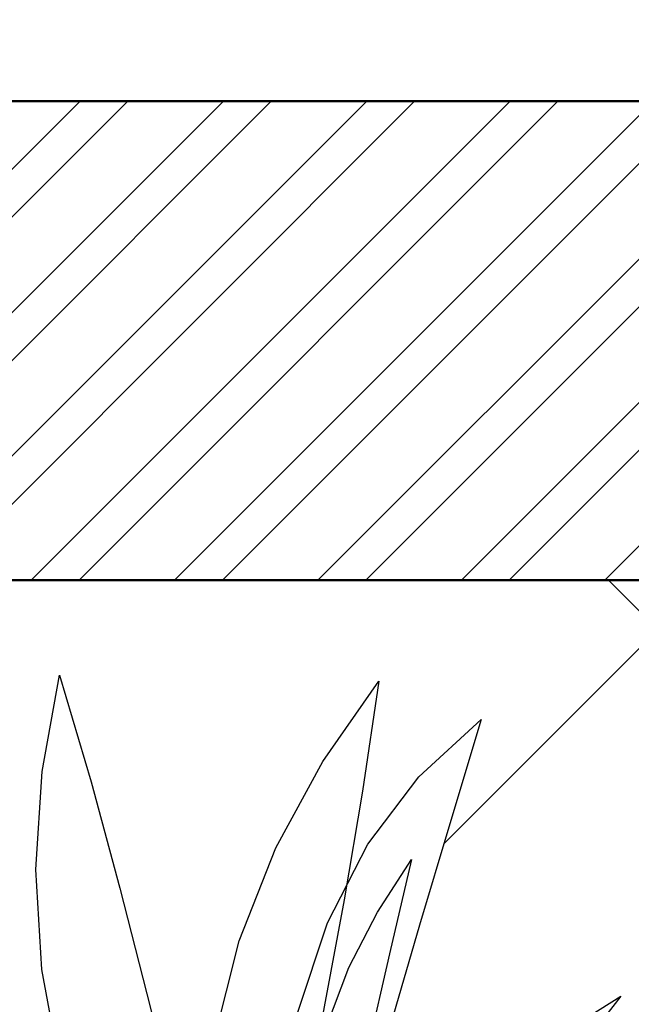
# Model space of a CAD drawing. Units: inches. Extents: x 3590 to 5167, y 65 to 1917.
# Tile 96 of 100: x 5045.84 to 5057.33, y 1789.03 to 1807.53. Entities that reach past the tile are written whole.
import ezdxf

# ---------------------------------------------------------------- set-up
doc = ezdxf.new("R2010")
doc.units = ezdxf.units.IN
for name, color, linetype, lineweight in [('A-ANNO-DIMS', 2, 'Continuous', 18), ('A-FLOR-PATT', 8, 'Continuous', 13), ('A-WALL', 7, 'Continuous', 50), ('A-WALL-PATT', 251, 'Continuous', 13), ('L-PLNT', 94, 'Continuous', 18)]:
    doc.layers.add(name, color=color, linetype=linetype, lineweight=lineweight)
doc.layers.add('DIENHOA', color=3, linetype='Continuous')
doc.styles.get("Standard").update_dxf_attribs({"font": 'arial.ttf'})
doc.dimstyles.new('ISO-25', dxfattribs={"dimtxt": 9, "dimasz": 2.5, "dimexe": 1.25, "dimexo": 0.625, "dimtad": 1, "dimdec": 1, "dimlunit": 3, "dimtxsty": 'Standard', "dimcen": 2.5, "dimadec": 0, "dimazin": 0, "dimtfac": 1, "dimtdec": 1, "dimtmove": 0, "dimatfit": 3, "dimfxl": 1, "dimarcsym": 0})

# ---------------------------------------------------------------- blocks, each defined once
blk = doc.blocks.new('*D101')
at = {"layer": 'A-ANNO-DIMS', "color": 0, "lineweight": -2, "transparency": 16777216}
for p, q in [((4420.274, 1806.624), (4420.274, 1818.615)), ((5080.274, 1806.624), (5080.274, 1818.615)), ((4422.774, 1817.365), (5077.774, 1817.365))]:
    blk.add_line(p, q, dxfattribs=at)
at = {"layer": 'A-ANNO-DIMS', "color": 0, "transparency": 16777216}
for points in [[(4422.774, 1817.781), (4422.774, 1816.948), (4420.274, 1817.365)], [(5077.774, 1817.781), (5077.774, 1816.948), (5080.274, 1817.365)]]:
    blk.add_solid(points, dxfattribs=at)
at = {"layer": 'Defpoints', "color": 0, "transparency": 16777216}
for p in [(5080.274, 1817.365), (4420.274, 1805.999), (5080.274, 1805.999)]:
    blk.add_point(p, dxfattribs=at)
at = {"layer": 'A-ANNO-DIMS', "color": 0, "transparency": 16777216, "insert": (4750.274, 1822.566), "char_height": 9, "attachment_point": 5}
blk.add_mtext("55'", dxfattribs=at)
blk = doc.blocks.new('Cay03_mb')
at = {"layer": 'DIENHOA'}
for p, q in [((118.58, 555.3), (166.15, 599.14)), ((166.15, 599.14), (142.15, 519.35)), ((79.49, 503.68), (118.58, 555.3)), ((142.15, 519.35), (118.96, 441.66)), ((48.56, 443.58), (79.49, 503.68)), ((25.49, 374.33), (48.56, 443.58)), ((118.96, 441.66), (96.72, 365.58))]:
    blk.add_line(p, q, dxfattribs=at)
for points in [[(23.69, -5.44), (-41, 82.2), (-91.83, 167.08), (-129.72, 249.45), (-155.55, 329.59), (-170.25, 407.76), (-174.71, 484.23), (-169.84, 559.26), (-156.54, 633.12)], [(-156.54, 633.12), (-132.46, 551.33), (-110.51, 470.02), (-89.84, 389.22), (-69.62, 308.98), (-48.99, 229.35), (-27.13, 150.38), (-3.18, 72.1), (23.69, -5.44)], [(-16.39, -26.73), (-38.34, 79.96), (-48.88, 178.33), (-48.7, 269), (-38.53, 352.58), (-19.08, 429.71), (8.95, 500.99), (44.86, 567.06), (87.92, 628.52)], [(87.92, 628.52), (75.46, 544.18), (61.27, 461.15), (46.13, 379.14), (30.83, 297.82), (16.14, 216.89), (2.85, 136.03), (-8.25, 54.92), (-16.39, -26.73)], [(23.69, -5.44), (19.84, 92.99), (20.28, 176.97), (25.02, 248.55), (34.03, 309.77), (47.33, 362.68), (64.91, 409.31), (86.75, 451.72), (112.87, 491.95)], [(112.87, 491.95), (95.99, 419.69), (79.46, 347.37), (63.92, 276.46), (50.01, 208.43), (38.38, 144.75), (29.69, 86.9), (24.57, 36.35), (23.69, -5.44)], [(273.24, 387.35), (227.6, 328.83), (182.25, 270.12), (138.39, 212.28), (97.23, 156.36), (59.96, 103.43), (27.8, 54.57), (1.94, 10.82), (-16.39, -26.73)], [(-16.39, -26.73), (21.41, 64.22), (57.05, 140.27), (91.37, 203.26), (125.24, 255.05), (159.51, 297.5), (195.03, 332.46), (232.65, 361.79), (273.24, 387.35)]]:
    blk.add_lwpolyline(points, dxfattribs=at)
blk = doc.blocks.new('*D323')
at = {"layer": 'A-ANNO-DIMS', "color": 0, "lineweight": -2, "transparency": 16777216}
for p, q in [((5069.172, 1795.216), (5069.172, 1874.95)), ((5065.437, 1795.216), (5070.422, 1795.216)), ((5069.172, 1769.309), (5069.172, 1792.716)), ((5065.437, 1766.809), (5070.422, 1766.809))]:
    blk.add_line(p, q, dxfattribs=at)
at = {"layer": 'A-ANNO-DIMS', "color": 0, "transparency": 16777216}
for points in [[(5068.756, 1792.716), (5069.589, 1792.716), (5069.172, 1795.216)], [(5068.756, 1769.309), (5069.589, 1769.309), (5069.172, 1766.809)]]:
    blk.add_solid(points, dxfattribs=at)
at = {"layer": 'Defpoints', "color": 0, "transparency": 16777216}
for p in [(5064.812, 1795.216), (5069.172, 1795.216), (5064.812, 1766.809)]:
    blk.add_point(p, dxfattribs=at)
at = {"layer": 'A-ANNO-DIMS', "color": 0, "transparency": 16777216, "insert": (5063.894, 1836.333), "char_height": 9, "attachment_point": 5, "rotation": 90}
blk.add_mtext('2\'-4 1/2" TYP.', dxfattribs=at)

msp = doc.modelspace()

# ---------------------------------------------------------------- hatches: boundary and pattern name
at = {"layer": 'A-FLOR-PATT', "transparency": 33554687}
h = msp.add_hatch(dxfattribs=at)
h.set_pattern_fill('AR-HBONE', color=256, scale=0.2)
h.set_pattern_definition([(45, (-588.972, 0), (0, 28.73682), [60.96, -20.32]), (135, (-574.604, 14.368), (3e-15, 28.73682), [60.96, -20.32])])
h.paths.add_polyline_path([(5071.274, 1796.999), (4933.274, 1796.999), (4933.274, 1753.999), (4962.774, 1753.999, -0.414214), (4928.774, 1719.999), (4933.274, 1718.999), (4933.274, 1334.999), (5071.274, 1334.999)])
h.paths.add_polyline_path([(4951.78, 1521.077), (4951.715, 1521.04), (4951.563, 1520.895)], flags=16)
h.paths.add_polyline_path([(4952.267, 1521.376), (4952.198, 1521.371), (4952.198, 1521.356)], flags=0)
h.paths.add_polyline_path([(4967.051, 1529.728), (4965.231, 1528.694), (4963.411, 1527.714), (4961.756, 1526.851), (4963.589, 1527.449), (4964.036, 1527.478), (4962.975, 1527.249), (4961.76, 1526.852), (4959.792, 1525.834), (4958.005, 1524.895), (4956.24, 1523.93), (4954.504, 1522.919), (4954.129, 1522.682), (4953.361, 1521.997), (4953.366, 1521.998), (4953.605, 1522.064), (4955.106, 1522.761), (4956.921, 1523.434), (4958.678, 1523.915), (4960.358, 1524.2), (4961.945, 1524.286), (4964.171, 1524.108), (4965.958, 1523.309), (4963.863, 1522.976), (4965.187, 1522.499), (4963.366, 1522.497), (4961.545, 1522.487), (4959.764, 1522.461), (4958.304, 1522.419), (4957.974, 1522.388), (4956.307, 1522.232), (4954.718, 1522.071), (4953.251, 1521.899), (4953.525, 1521.623), (4954.331, 1521.379), (4956.243, 1521.23), (4958.039, 1520.93), (4959.684, 1520.483), (4961.16, 1519.896), (4963.107, 1518.8), (4964.393, 1517.325), (4962.973, 1517.726), (4964.558, 1516.661), (4965.407, 1515.708), (4963.507, 1516.322), (4961.68, 1517.005), (4959.935, 1517.745), (4958.282, 1518.528), (4956.732, 1519.343), (4955.295, 1520.175), (4954.672, 1520.572), (4954.513, 1520.627), (4955.658, 1519.318), (4956.703, 1517.982), (4957.644, 1516.647), (4958.485, 1515.334), (4959.55, 1513.524), (4960.438, 1511.769), (4958.841, 1513.62), (4957.452, 1515.325), (4955.819, 1517.459), (4956.665, 1515.448), (4957.111, 1513.923), (4957.447, 1511.714), (4957.076, 1509.793), (4956.538, 1511.11), (4955.992, 1512.569), (4955.444, 1514.125), (4954.898, 1515.735), (4954.357, 1517.356), (4953.824, 1518.943), (4953.305, 1520.452), (4953.065, 1521.116), (4952.971, 1521.146), (4952.949, 1521.086), (4952.73, 1520.199), (4953.37, 1518.024), (4953.757, 1516.373), (4954.051, 1514.765), (4954.264, 1513.221), (4954.471, 1511.131), (4954.497, 1510.402), (4954.409, 1511.76), (4954.264, 1513.221), (4954.051, 1514.765), (4953.757, 1516.373), (4953.37, 1518.024), (4952.877, 1519.698), (4952.716, 1520.141), (4952.533, 1519.059), (4952.374, 1517.789), (4952.219, 1516.312), (4952.046, 1514.6), (4951.833, 1512.626), (4951.557, 1510.363), (4951.203, 1512.168), (4950.852, 1514.339), (4950.985, 1516.376), (4951.66, 1518.286), (4952.593, 1520.481), (4952.357, 1521.13), (4951.855, 1520.328), (4950.839, 1518.908), (4949.777, 1517.587), (4948.916, 1516.617), (4948.111, 1515.256), (4947.089, 1513.554), (4945.889, 1511.615), (4946.326, 1513.402), (4946.562, 1514.249), (4945.528, 1513.327), (4944.581, 1512.531), (4946.018, 1514.508), (4947.204, 1516.048), (4947.893, 1517.313), (4949.307, 1518.764), (4950.414, 1519.767), (4950.451, 1519.806), (4952.267, 1521.376), (4951.645, 1521.493), (4950.404, 1521.18), (4948.044, 1520.359), (4946.119, 1519.452), (4944.572, 1518.475), (4943.35, 1517.443), (4941.997, 1515.92), (4941.661, 1515.275), (4942.813, 1516.99), (4944.572, 1518.475), (4946.119, 1519.452), (4948.044, 1520.359), (4950.404, 1521.18), (4951.645, 1521.493), (4949.647, 1521.868), (4948.6, 1521.756), (4947.126, 1521.57), (4945.42, 1521.348), (4943.45, 1521.105), (4941.183, 1520.856), (4942.86, 1521.613), (4943.873, 1522.03), (4942.952, 1521.909), (4941.41, 1521.485), (4939.543, 1520.67), (4938.968, 1520.226), (4940.733, 1521.299), (4942.952, 1521.909), (4943.702, 1522.008), (4945.894, 1522.7), (4947.565, 1522.714), (4948.921, 1522.566), (4951.131, 1522.183), (4950.971, 1522.297), (4948.129, 1523.006), (4946.035, 1523.707), (4944.232, 1524.521), (4942.707, 1525.461), (4941.444, 1526.537), (4940.43, 1527.761), (4939.649, 1529.143), (4941.421, 1528.122), (4943.147, 1527.132), (4944.841, 1526.175), (4946.514, 1525.25), (4948.179, 1524.359), (4948.365, 1524.263), (4946.475, 1526.045), (4945.181, 1527.54), (4944.19, 1529.033), (4943.496, 1530.54), (4943.278, 1531.36), (4942.498, 1531.919), (4943.114, 1531.762), (4942.959, 1533.659), (4944.14, 1531.989), (4944.612, 1531.323), (4946.202, 1530.463), (4947.486, 1529.509), (4948.79, 1528.226), (4950.368, 1526.237), (4949.485, 1528.155), (4948.851, 1530.123), (4948.491, 1532.041), (4948.381, 1533.918), (4948.501, 1535.76), (4948.827, 1537.573), (4949.418, 1535.565), (4949.957, 1533.569), (4950.464, 1531.586), (4950.961, 1529.617), (4951.391, 1527.954), (4951.724, 1530.687), (4952.201, 1532.58), (4952.889, 1534.33), (4953.77, 1535.951), (4954.827, 1537.46), (4954.521, 1535.39), (4954.273, 1533.937), (4955.58, 1535.663), (4956.748, 1536.739), (4956.159, 1534.78), (4955.589, 1532.873), (4955.043, 1531.006), (4954.525, 1529.166), (4954.038, 1527.341), (4953.638, 1525.733), (4953.611, 1525.586), (4953.398, 1524.166), (4953.382, 1524.009), (4954.07, 1525.476), (4954.912, 1527.022), (4956.136, 1528.894), (4957.847, 1530.577), (4959.376, 1531.54), (4958.256, 1530.104), (4957.143, 1528.663), (4956.066, 1527.243), (4955.056, 1525.871), (4954.141, 1524.571), (4953.352, 1523.372), (4953.311, 1523.303), (4953.273, 1522.925), (4953.261, 1522.382), (4954.103, 1523.373), (4954.63, 1524.284), (4955.961, 1526.358), (4957.23, 1528.13), (4958.421, 1529.609), (4960.037, 1531.368), (4961.374, 1532.375), (4962.101, 1532.77), (4961.07, 1531.061), (4959.987, 1529.438), (4958.869, 1527.908), (4958.15, 1527.007), (4959.803, 1528.003), (4961.589, 1528.793), (4963.391, 1529.328), (4965.211, 1529.632)], flags=16)
h.paths.add_polyline_path([(4962.944, 1523.182), (4961.107, 1523.422), (4960.392, 1523.362), (4962.35, 1523.331)], flags=0)
h.paths.add_polyline_path([(5049.541, 1584.551), (5049.476, 1584.515), (5049.325, 1584.37)], flags=16)
h.paths.add_polyline_path([(5050.028, 1584.851), (5049.959, 1584.845), (5049.959, 1584.83)], flags=0)
h.paths.add_polyline_path([(5042.333, 1581.949), (5043.88, 1582.926), (5045.806, 1583.833), (5048.165, 1584.654), (5049.406, 1584.967), (5047.408, 1585.342), (5046.361, 1585.231), (5044.888, 1585.044), (5043.181, 1584.822), (5041.211, 1584.579), (5038.944, 1584.33), (5040.622, 1585.087), (5041.634, 1585.504), (5040.713, 1585.383), (5039.171, 1584.959), (5037.304, 1584.144), (5036.729, 1583.7), (5038.494, 1584.773), (5040.713, 1585.383), (5041.463, 1585.482), (5043.655, 1586.174), (5045.326, 1586.188), (5046.682, 1586.04), (5048.893, 1585.657), (5048.732, 1585.771), (5045.891, 1586.48), (5043.796, 1587.181), (5041.994, 1587.996), (5040.468, 1588.935), (5039.205, 1590.011), (5038.191, 1591.235), (5037.41, 1592.617), (5039.182, 1591.596), (5040.909, 1590.607), (5042.602, 1589.649), (5044.275, 1588.724), (5045.94, 1587.833), (5046.126, 1587.738), (5044.237, 1589.519), (5042.942, 1591.015), (5041.952, 1592.508), (5041.257, 1594.014), (5041.039, 1594.834), (5040.26, 1595.393), (5040.875, 1595.237), (5040.721, 1597.133), (5041.901, 1595.463), (5042.373, 1594.798), (5043.963, 1593.938), (5045.247, 1592.983), (5046.552, 1591.701), (5048.129, 1589.712), (5047.247, 1591.63), (5046.613, 1593.597), (5046.252, 1595.515), (5046.142, 1597.392), (5046.262, 1599.234), (5046.588, 1601.047), (5047.179, 1599.039), (5047.718, 1597.043), (5048.225, 1595.06), (5048.722, 1593.091), (5049.152, 1591.429), (5049.485, 1594.161), (5049.962, 1596.054), (5050.65, 1597.804), (5051.532, 1599.425), (5052.589, 1600.934), (5052.283, 1598.864), (5052.034, 1597.411), (5053.341, 1599.137), (5054.509, 1600.213), (5053.92, 1598.254), (5053.35, 1596.348), (5052.805, 1594.48), (5052.286, 1592.64), (5051.799, 1590.815), (5051.4, 1589.207), (5051.373, 1589.06), (5051.159, 1587.64), (5051.143, 1587.483), (5051.831, 1588.95), (5052.673, 1590.496), (5053.898, 1592.368), (5055.608, 1594.051), (5057.137, 1595.014), (5056.017, 1593.578), (5054.904, 1592.137), (5053.828, 1590.717), (5052.817, 1589.345), (5051.902, 1588.046), (5051.113, 1586.846), (5051.072, 1586.777), (5051.034, 1586.399), (5051.022, 1585.856), (5051.864, 1586.847), (5052.391, 1587.758), (5053.723, 1589.832), (5054.991, 1591.604), (5056.182, 1593.083), (5057.798, 1594.842), (5059.135, 1595.849), (5059.863, 1596.244), (5058.831, 1594.535), (5057.749, 1592.912), (5056.63, 1591.382), (5055.912, 1590.482), (5057.564, 1591.477), (5059.35, 1592.267), (5061.152, 1592.802), (5062.972, 1593.106), (5064.812, 1593.203), (5062.992, 1592.169), (5061.172, 1591.188), (5059.518, 1590.325), (5061.35, 1590.924), (5061.797, 1590.952), (5060.737, 1590.723), (5059.521, 1590.326), (5057.553, 1589.308), (5055.766, 1588.369), (5054.002, 1587.404), (5052.265, 1586.393), (5051.891, 1586.156), (5051.122, 1585.471), (5051.127, 1585.472), (5051.366, 1585.538), (5052.867, 1586.235), (5054.682, 1586.908), (5056.439, 1587.389), (5058.12, 1587.675), (5059.706, 1587.76), (5061.933, 1587.583), (5063.719, 1586.783), (5061.624, 1586.45), (5062.949, 1585.973), (5061.127, 1585.971), (5059.307, 1585.961), (5057.525, 1585.935), (5056.065, 1585.893), (5055.735, 1585.862), (5054.068, 1585.707), (5052.479, 1585.546), (5051.012, 1585.373), (5051.286, 1585.097), (5052.092, 1584.853), (5054.004, 1584.704), (5055.8, 1584.404), (5057.446, 1583.958), (5058.921, 1583.37), (5060.868, 1582.274), (5062.154, 1580.799), (5060.734, 1581.2), (5062.32, 1580.135), (5063.168, 1579.182), (5061.269, 1579.796), (5059.441, 1580.479), (5057.696, 1581.219), (5056.043, 1582.003), (5054.493, 1582.817), (5053.057, 1583.649), (5052.433, 1584.047), (5052.274, 1584.101), (5053.42, 1582.793), (5054.464, 1581.457), (5055.405, 1580.121), (5056.247, 1578.809), (5057.311, 1576.998), (5058.199, 1575.244), (5056.602, 1577.094), (5055.213, 1578.799), (5053.58, 1580.933), (5054.427, 1578.922), (5054.872, 1577.397), (5055.208, 1575.189), (5054.838, 1573.267), (5054.299, 1574.584), (5053.754, 1576.043), (5053.206, 1577.599), (5052.659, 1579.209), (5052.118, 1580.83), (5051.585, 1582.417), (5051.066, 1583.927), (5050.826, 1584.59), (5050.733, 1584.62), (5050.711, 1584.561), (5050.491, 1583.673), (5051.131, 1581.498), (5051.518, 1579.847), (5051.813, 1578.24), (5052.026, 1576.695), (5052.233, 1574.605), (5052.258, 1573.876), (5052.17, 1575.234), (5052.026, 1576.695), (5051.813, 1578.24), (5051.518, 1579.847), (5051.131, 1581.498), (5050.638, 1583.172), (5050.477, 1583.615), (5050.294, 1582.533), (5050.136, 1581.263), (5049.981, 1579.786), (5049.807, 1578.074), (5049.594, 1576.1), (5049.318, 1573.837), (5048.965, 1575.642), (5048.613, 1577.813), (5048.747, 1579.85), (5049.421, 1581.76), (5050.354, 1583.955), (5050.118, 1584.604), (5049.616, 1583.802), (5048.6, 1582.382), (5047.538, 1581.061), (5046.677, 1580.091), (5045.872, 1578.73), (5044.85, 1577.028), (5043.651, 1575.089), (5044.087, 1576.877), (5044.324, 1577.723), (5043.289, 1576.801), (5042.342, 1576.005), (5043.779, 1577.982), (5044.966, 1579.522), (5045.655, 1580.787), (5047.068, 1582.239), (5048.175, 1583.241), (5048.213, 1583.28), (5050.028, 1584.851), (5049.406, 1584.967), (5048.165, 1584.654), (5045.806, 1583.833), (5043.88, 1582.926), (5042.333, 1581.949), (5041.111, 1580.917), (5039.758, 1579.394), (5039.423, 1578.749), (5040.575, 1580.464)], flags=16)
h.paths.add_polyline_path([(4954.799, 1533.12), (4954.262, 1532.079), (4953.831, 1530.935), (4953.505, 1529.636), (4953.283, 1528.133), (4953.167, 1526.376), (4953.156, 1524.315), (4953.277, 1521.236), (4952.802, 1521.842), (4951.557, 1521.998), (4950.976, 1521.961), (4952.661, 1521.941), (4952.802, 1521.842), (4953.152, 1523.593), (4953.167, 1526.376), (4953.283, 1528.133), (4953.609, 1530.346), (4954.456, 1532.592)], flags=0)
h.paths.add_polyline_path([(5050.563, 1585.316), (5049.318, 1585.472), (5048.737, 1585.435), (5050.422, 1585.415), (5050.563, 1585.316), (5050.914, 1587.067), (5050.928, 1589.851), (5051.045, 1591.607), (5051.371, 1593.82), (5052.217, 1596.066), (5052.56, 1596.594), (5052.024, 1595.554), (5051.592, 1594.409), (5051.266, 1593.11), (5051.045, 1591.607), (5050.928, 1589.851), (5050.918, 1587.789), (5051.038, 1584.71)], flags=0)
h.paths.add_polyline_path([(5058.153, 1586.836), (5060.111, 1586.805), (5060.705, 1586.656), (5058.868, 1586.896)], flags=0)
h.paths.add_polyline_path([(5049.541, 1430.936), (5049.476, 1430.9), (5049.325, 1430.755)], flags=16)
h.paths.add_polyline_path([(5050.028, 1431.236), (5049.959, 1431.231), (5049.959, 1431.215)], flags=0)
h.paths.add_polyline_path([(5046.588, 1447.432), (5047.179, 1445.425), (5047.718, 1443.429), (5048.225, 1441.446), (5048.722, 1439.476), (5049.152, 1437.814), (5049.485, 1440.546), (5049.962, 1442.439), (5050.65, 1444.189), (5051.532, 1445.811), (5052.589, 1447.319), (5052.283, 1445.249), (5052.034, 1443.796), (5053.341, 1445.522), (5054.509, 1446.598), (5053.92, 1444.64), (5053.35, 1442.733), (5052.805, 1440.865), (5052.286, 1439.025), (5051.799, 1437.201), (5051.4, 1435.592), (5051.373, 1435.445), (5051.159, 1434.025), (5051.143, 1433.868), (5051.831, 1435.335), (5052.673, 1436.881), (5053.898, 1438.753), (5055.608, 1440.436), (5057.137, 1441.4), (5056.017, 1439.963), (5054.904, 1438.522), (5053.828, 1437.102), (5052.817, 1435.73), (5051.902, 1434.431), (5051.113, 1433.231), (5051.072, 1433.162), (5051.034, 1432.784), (5051.022, 1432.242), (5051.864, 1433.232), (5052.391, 1434.143), (5053.723, 1436.217), (5054.991, 1437.989), (5056.182, 1439.468), (5057.798, 1441.227), (5059.135, 1442.235), (5059.863, 1442.629), (5058.831, 1440.921), (5057.749, 1439.298), (5056.63, 1437.767), (5055.912, 1436.867), (5057.564, 1437.863), (5059.35, 1438.652), (5061.152, 1439.187), (5062.972, 1439.491), (5064.812, 1439.588), (5062.992, 1438.554), (5061.172, 1437.573), (5059.518, 1436.71), (5061.35, 1437.309), (5061.797, 1437.337), (5060.737, 1437.108), (5059.521, 1436.711), (5057.553, 1435.693), (5055.766, 1434.754), (5054.002, 1433.789), (5052.265, 1432.778), (5051.891, 1432.541), (5051.122, 1431.856), (5051.127, 1431.857), (5051.366, 1431.923), (5052.867, 1432.62), (5054.682, 1433.293), (5056.439, 1433.775), (5058.12, 1434.06), (5059.706, 1434.145), (5061.933, 1433.968), (5063.719, 1433.168), (5061.624, 1432.835), (5062.949, 1432.358), (5061.127, 1432.357), (5059.307, 1432.346), (5057.525, 1432.32), (5056.065, 1432.278), (5055.735, 1432.248), (5054.068, 1432.092), (5052.479, 1431.931), (5051.012, 1431.759), (5051.286, 1431.482), (5052.092, 1431.238), (5054.004, 1431.089), (5055.8, 1430.789), (5057.446, 1430.343), (5058.921, 1429.755), (5060.868, 1428.66), (5062.154, 1427.185), (5060.734, 1427.585), (5062.32, 1426.52), (5063.168, 1425.567), (5061.269, 1426.181), (5059.441, 1426.865), (5057.696, 1427.604), (5056.043, 1428.388), (5054.493, 1429.202), (5053.057, 1430.034), (5052.433, 1430.432), (5052.274, 1430.487), (5053.42, 1429.178), (5054.464, 1427.842), (5055.405, 1426.506), (5056.247, 1425.194), (5057.311, 1423.383), (5058.199, 1421.629), (5056.602, 1423.479), (5055.213, 1425.184), (5053.58, 1427.318), (5054.427, 1425.307), (5054.872, 1423.782), (5055.208, 1421.574), (5054.838, 1419.652), (5054.299, 1420.97), (5053.754, 1422.428), (5053.206, 1423.984), (5052.659, 1425.595), (5052.118, 1427.215), (5051.585, 1428.802), (5051.066, 1430.312), (5050.826, 1430.975), (5050.733, 1431.005), (5050.711, 1430.946), (5050.491, 1430.058), (5051.131, 1427.883), (5051.518, 1426.232), (5051.813, 1424.625), (5052.026, 1423.081), (5052.233, 1420.991), (5052.258, 1420.261), (5052.17, 1421.619), (5052.026, 1423.081), (5051.813, 1424.625), (5051.518, 1426.232), (5051.131, 1427.883), (5050.638, 1429.558), (5050.477, 1430.001), (5050.294, 1428.918), (5050.136, 1427.648), (5049.981, 1426.171), (5049.807, 1424.459), (5049.594, 1422.485), (5049.318, 1420.222), (5048.965, 1422.028), (5048.613, 1424.199), (5048.747, 1426.235), (5049.421, 1428.146), (5050.354, 1430.34), (5050.118, 1430.989), (5049.616, 1430.187), (5048.6, 1428.768), (5047.538, 1427.446), (5046.677, 1426.477), (5045.872, 1425.116), (5044.85, 1423.413), (5043.651, 1421.474), (5044.087, 1423.262), (5044.324, 1424.109), (5043.289, 1423.186), (5042.342, 1422.391), (5043.779, 1424.368), (5044.966, 1425.907), (5045.655, 1427.173), (5047.068, 1428.624), (5048.175, 1429.627), (5048.213, 1429.666), (5050.028, 1431.236), (5049.406, 1431.353), (5048.165, 1431.039), (5045.806, 1430.218), (5043.88, 1429.311), (5042.333, 1428.334), (5041.111, 1427.302), (5039.758, 1425.779), (5039.423, 1425.134), (5040.575, 1426.849), (5042.333, 1428.334), (5043.88, 1429.311), (5045.806, 1430.218), (5048.165, 1431.039), (5049.406, 1431.353), (5047.408, 1431.727), (5046.361, 1431.616), (5044.888, 1431.429), (5043.181, 1431.207), (5041.211, 1430.964), (5038.944, 1430.715), (5040.622, 1431.472), (5041.634, 1431.89), (5040.713, 1431.769), (5039.171, 1431.345), (5037.304, 1430.53), (5036.729, 1430.085), (5038.494, 1431.158), (5040.713, 1431.769), (5041.463, 1431.867), (5043.655, 1432.559), (5045.326, 1432.573), (5046.682, 1432.425), (5048.893, 1432.042), (5048.732, 1432.156), (5045.891, 1432.865), (5043.796, 1433.566), (5041.994, 1434.381), (5040.468, 1435.321), (5039.205, 1436.396), (5038.191, 1437.62), (5037.41, 1439.002), (5039.182, 1437.982), (5040.909, 1436.992), (5042.602, 1436.034), (5044.275, 1435.109), (5045.94, 1434.218), (5046.126, 1434.123), (5044.237, 1435.904), (5042.942, 1437.4), (5041.952, 1438.893), (5041.257, 1440.399), (5041.039, 1441.219), (5040.26, 1441.778), (5040.875, 1441.622), (5040.721, 1443.518), (5041.901, 1441.848), (5042.373, 1441.183), (5043.963, 1440.323), (5045.247, 1439.369), (5046.552, 1438.086), (5048.129, 1436.097), (5047.247, 1438.015), (5046.613, 1439.982), (5046.252, 1441.901), (5046.142, 1443.778), (5046.262, 1445.619)], flags=16)
h.paths.add_polyline_path([(5052.382, 1444.255), (5051.623, 1442.78), (5052.024, 1441.939), (5052.56, 1442.98)], flags=0)
h.paths.add_polyline_path([(5050.563, 1431.701), (5049.318, 1431.857), (5048.737, 1431.821), (5050.422, 1431.8)], flags=0)
h.paths.add_polyline_path([(5058.153, 1433.221), (5060.111, 1433.19), (5060.705, 1433.041), (5058.868, 1433.281)], flags=0)
h.paths.add_polyline_path([(5049.541, 1352.285), (5049.476, 1352.249), (5049.325, 1352.104)], flags=16)
h.paths.add_polyline_path([(5050.028, 1352.585), (5049.959, 1352.58), (5049.959, 1352.564)], flags=0)
h.paths.add_polyline_path([(5046.588, 1368.781), (5047.179, 1366.774), (5047.718, 1364.778), (5048.225, 1362.795), (5048.722, 1360.825), (5049.152, 1359.163), (5049.485, 1361.896), (5049.962, 1363.789), (5050.65, 1365.538), (5051.532, 1367.16), (5052.589, 1368.669), (5052.283, 1366.598), (5052.034, 1365.145), (5053.341, 1366.871), (5054.509, 1367.947), (5053.92, 1365.989), (5053.35, 1364.082), (5052.805, 1362.214), (5052.286, 1360.374), (5051.799, 1358.55), (5051.4, 1356.942), (5051.373, 1356.794), (5051.159, 1355.374), (5051.143, 1355.218), (5051.831, 1356.684), (5052.673, 1358.23), (5053.898, 1360.102), (5055.608, 1361.786), (5057.137, 1362.749), (5056.017, 1361.313), (5054.904, 1359.872), (5053.828, 1358.452), (5052.817, 1357.079), (5051.902, 1355.78), (5051.113, 1354.581), (5051.072, 1354.512), (5051.034, 1354.133), (5051.022, 1353.591), (5051.864, 1354.581), (5052.391, 1355.492), (5053.723, 1357.566), (5054.991, 1359.338), (5056.182, 1360.817), (5057.798, 1362.577), (5059.135, 1363.584), (5059.863, 1363.979), (5058.831, 1362.27), (5057.749, 1360.647), (5056.63, 1359.117), (5055.912, 1358.216), (5057.564, 1359.212), (5059.35, 1360.001), (5061.152, 1360.536), (5062.972, 1360.841), (5064.812, 1360.937), (5062.992, 1359.903), (5061.172, 1358.923), (5059.518, 1358.059), (5061.35, 1358.658), (5061.797, 1358.687), (5060.737, 1358.458), (5059.521, 1358.061), (5057.553, 1357.043), (5055.766, 1356.103), (5054.002, 1355.138), (5052.265, 1354.127), (5051.891, 1353.89), (5051.122, 1353.206), (5051.127, 1353.206), (5051.366, 1353.272), (5052.867, 1353.969), (5054.682, 1354.643), (5056.439, 1355.124), (5058.12, 1355.409), (5059.706, 1355.495), (5061.933, 1355.317), (5063.719, 1354.518), (5061.624, 1354.184), (5062.949, 1353.708), (5061.127, 1353.706), (5059.307, 1353.695), (5057.525, 1353.669), (5056.065, 1353.627), (5055.735, 1353.597), (5054.068, 1353.441), (5052.479, 1353.28), (5051.012, 1353.108), (5051.286, 1352.831), (5052.092, 1352.587), (5054.004, 1352.439), (5055.8, 1352.138), (5057.446, 1351.692), (5058.921, 1351.104), (5060.868, 1350.009), (5062.154, 1348.534), (5060.734, 1348.935), (5062.32, 1347.869), (5063.168, 1346.916), (5061.269, 1347.53), (5059.441, 1348.214), (5057.696, 1348.954), (5056.043, 1349.737), (5054.493, 1350.551), (5053.057, 1351.383), (5052.433, 1351.781), (5052.274, 1351.836), (5053.42, 1350.527), (5054.464, 1349.191), (5055.405, 1347.855), (5056.247, 1346.543), (5057.311, 1344.733), (5058.199, 1342.978), (5056.602, 1344.828), (5055.213, 1346.534), (5053.58, 1348.667), (5054.427, 1346.656), (5054.872, 1345.132), (5055.208, 1342.923), (5054.838, 1341.002), (5054.299, 1342.319), (5053.754, 1343.778), (5053.206, 1345.334), (5052.659, 1346.944), (5052.118, 1348.564), (5051.585, 1350.151), (5051.066, 1351.661), (5050.826, 1352.324), (5050.733, 1352.355), (5050.711, 1352.295), (5050.491, 1351.408), (5051.131, 1349.232), (5051.518, 1347.581), (5051.813, 1345.974), (5052.026, 1344.43), (5052.233, 1342.34), (5052.258, 1341.61), (5052.17, 1342.969), (5052.026, 1344.43), (5051.813, 1345.974), (5051.518, 1347.581), (5051.131, 1349.232), (5050.638, 1350.907), (5050.477, 1351.35), (5050.294, 1350.267), (5050.136, 1348.997), (5049.981, 1347.52), (5049.807, 1345.809), (5049.594, 1343.835), (5049.318, 1341.571), (5048.965, 1343.377), (5048.613, 1345.548), (5048.747, 1347.585), (5049.421, 1349.495), (5050.354, 1351.689), (5050.118, 1352.339), (5049.616, 1351.536), (5048.6, 1350.117), (5047.538, 1348.795), (5046.677, 1347.826), (5045.872, 1346.465), (5044.85, 1344.763), (5043.651, 1342.824), (5044.087, 1344.611), (5044.324, 1345.458), (5043.289, 1344.535), (5042.342, 1343.74), (5043.779, 1345.717), (5044.966, 1347.256), (5045.655, 1348.522), (5047.068, 1349.973), (5048.175, 1350.976), (5048.213, 1351.015), (5050.028, 1352.585), (5049.406, 1352.702), (5048.165, 1352.388), (5045.806, 1351.567), (5043.88, 1350.661), (5042.333, 1349.683), (5041.111, 1348.651), (5039.758, 1347.128), (5039.423, 1346.483), (5040.575, 1348.198), (5042.333, 1349.683), (5043.88, 1350.661), (5045.806, 1351.567), (5048.165, 1352.388), (5049.406, 1352.702), (5047.408, 1353.076), (5046.361, 1352.965), (5044.888, 1352.779), (5043.181, 1352.556), (5041.211, 1352.313), (5038.944, 1352.065), (5040.622, 1352.821), (5041.634, 1353.239), (5040.713, 1353.118), (5039.171, 1352.694), (5037.304, 1351.879), (5036.729, 1351.434), (5038.494, 1352.508), (5040.713, 1353.118), (5041.463, 1353.216), (5043.655, 1353.909), (5045.326, 1353.923), (5046.682, 1353.774), (5048.893, 1353.391), (5048.732, 1353.506), (5045.891, 1354.214), (5043.796, 1354.915), (5041.994, 1355.73), (5040.468, 1356.67), (5039.205, 1357.746), (5038.191, 1358.969), (5037.41, 1360.352), (5039.182, 1359.331), (5040.909, 1358.341), (5042.602, 1357.383), (5044.275, 1356.458), (5045.94, 1355.567), (5046.126, 1355.472), (5044.237, 1357.253), (5042.942, 1358.749), (5041.952, 1360.242), (5041.257, 1361.748), (5041.039, 1362.568), (5040.26, 1363.128), (5040.875, 1362.971), (5040.721, 1364.867), (5041.901, 1363.197), (5042.373, 1362.532), (5043.963, 1361.672), (5045.247, 1360.718), (5046.552, 1359.435), (5048.129, 1357.446), (5047.247, 1359.364), (5046.613, 1361.331), (5046.252, 1363.25), (5046.142, 1365.127), (5046.262, 1366.969)], flags=16)
h.paths.add_polyline_path([(5052.382, 1365.604), (5051.623, 1364.129), (5052.024, 1363.288), (5052.56, 1364.329)], flags=0)
h.paths.add_polyline_path([(4951.78, 1698.041), (4951.715, 1698.005), (4951.563, 1697.859)], flags=16)
h.paths.add_polyline_path([(4952.267, 1698.341), (4952.198, 1698.335), (4952.198, 1698.32)], flags=0)
h.paths.add_polyline_path([(4957.076, 1686.757), (4956.538, 1688.074), (4955.992, 1689.533), (4955.444, 1691.089), (4954.898, 1692.699), (4954.357, 1694.32), (4953.824, 1695.907), (4953.305, 1697.417), (4953.065, 1698.08), (4952.971, 1698.11), (4952.949, 1698.051), (4952.73, 1697.163), (4953.37, 1694.988), (4953.757, 1693.337), (4954.051, 1691.729), (4954.264, 1690.185), (4954.471, 1688.095), (4954.497, 1687.366), (4954.409, 1688.724), (4954.264, 1690.185), (4954.051, 1691.729), (4953.757, 1693.337), (4953.37, 1694.988), (4952.877, 1696.662), (4952.716, 1697.105), (4952.533, 1696.023), (4952.374, 1694.753), (4952.219, 1693.276), (4952.046, 1691.564), (4951.833, 1689.59), (4951.557, 1687.327), (4951.203, 1689.132), (4950.852, 1691.303), (4950.985, 1693.34), (4951.66, 1695.25), (4952.593, 1697.445), (4952.357, 1698.094), (4951.855, 1697.292), (4950.839, 1695.872), (4949.777, 1694.551), (4948.916, 1693.581), (4948.111, 1692.22), (4947.089, 1690.518), (4945.889, 1688.579), (4946.326, 1690.366), (4946.562, 1691.213), (4945.528, 1690.291), (4944.581, 1689.495), (4946.018, 1691.472), (4947.204, 1693.012), (4947.893, 1694.277), (4949.307, 1695.729), (4950.414, 1696.731), (4950.451, 1696.77), (4952.267, 1698.341), (4951.645, 1698.457), (4950.404, 1698.144), (4948.044, 1697.323), (4946.119, 1696.416), (4944.572, 1695.439), (4943.35, 1694.407), (4941.997, 1692.884), (4941.661, 1692.239), (4942.813, 1693.954), (4944.572, 1695.439), (4946.119, 1696.416), (4948.044, 1697.323), (4950.404, 1698.144), (4951.645, 1698.457), (4949.647, 1698.832), (4948.6, 1698.72), (4947.126, 1698.534), (4945.42, 1698.312), (4943.45, 1698.069), (4941.183, 1697.82), (4942.86, 1698.577), (4943.873, 1698.994), (4942.952, 1698.873), (4941.41, 1698.449), (4939.543, 1697.634), (4938.968, 1697.19), (4940.733, 1698.263), (4942.952, 1698.873), (4943.702, 1698.972), (4945.894, 1699.664), (4947.565, 1699.678), (4948.921, 1699.53), (4951.131, 1699.147), (4950.971, 1699.261), (4948.129, 1699.97), (4946.035, 1700.671), (4944.232, 1701.486), (4942.707, 1702.425), (4941.444, 1703.501), (4940.43, 1704.725), (4939.649, 1706.107), (4941.421, 1705.086), (4943.147, 1704.097), (4944.841, 1703.139), (4946.514, 1702.214), (4948.179, 1701.323), (4948.365, 1701.227), (4946.475, 1703.009), (4945.181, 1704.505), (4944.19, 1705.997), (4943.496, 1707.504), (4943.278, 1708.324), (4942.498, 1708.883), (4943.114, 1708.727), (4942.959, 1710.623), (4944.14, 1708.953), (4944.612, 1708.287), (4946.202, 1707.428), (4947.486, 1706.473), (4948.79, 1705.191), (4950.368, 1703.202), (4949.485, 1705.12), (4948.851, 1707.087), (4948.491, 1709.005), (4948.381, 1710.882), (4948.501, 1712.724), (4948.827, 1714.537), (4949.418, 1712.529), (4949.957, 1710.533), (4950.464, 1708.55), (4950.961, 1706.581), (4951.391, 1704.919), (4951.724, 1707.651), (4952.201, 1709.544), (4952.889, 1711.294), (4953.77, 1712.915), (4954.827, 1714.424), (4954.521, 1712.354), (4954.273, 1710.901), (4955.58, 1712.627), (4956.748, 1713.703), (4956.159, 1711.744), (4955.589, 1709.837), (4955.043, 1707.97), (4954.525, 1706.13), (4954.038, 1704.305), (4953.638, 1702.697), (4953.611, 1702.55), (4953.398, 1701.13), (4953.382, 1700.973), (4954.07, 1702.44), (4954.912, 1703.986), (4956.136, 1705.858), (4957.847, 1707.541), (4959.376, 1708.504), (4958.256, 1707.068), (4957.143, 1705.627), (4956.066, 1704.207), (4955.056, 1702.835), (4954.141, 1701.536), (4953.352, 1700.336), (4953.311, 1700.267), (4953.273, 1699.889), (4953.261, 1699.346), (4954.103, 1700.337), (4954.63, 1701.248), (4955.961, 1703.322), (4957.23, 1705.094), (4958.421, 1706.573), (4960.037, 1708.332), (4961.374, 1709.339), (4962.101, 1709.734), (4961.07, 1708.025), (4959.987, 1706.402), (4958.869, 1704.872), (4958.15, 1703.972), (4959.803, 1704.967), (4961.589, 1705.757), (4963.391, 1706.292), (4965.211, 1706.596), (4967.051, 1706.692), (4965.231, 1705.659), (4963.411, 1704.678), (4961.756, 1703.815), (4963.589, 1704.413), (4964.036, 1704.442), (4962.975, 1704.213), (4961.76, 1703.816), (4959.792, 1702.798), (4958.005, 1701.859), (4956.24, 1700.894), (4954.504, 1699.883), (4954.129, 1699.646), (4953.361, 1698.961), (4953.366, 1698.962), (4953.605, 1699.028), (4955.106, 1699.725), (4956.921, 1700.398), (4958.678, 1700.879), (4960.358, 1701.164), (4961.945, 1701.25), (4964.171, 1701.073), (4965.958, 1700.273), (4963.863, 1699.94), (4965.187, 1699.463), (4963.366, 1699.461), (4961.545, 1699.451), (4959.764, 1699.425), (4958.304, 1699.383), (4957.974, 1699.352), (4956.307, 1699.197), (4954.718, 1699.036), (4953.251, 1698.863), (4953.525, 1698.587), (4954.331, 1698.343), (4956.243, 1698.194), (4958.039, 1697.894), (4959.684, 1697.447), (4961.16, 1696.86), (4963.107, 1695.764), (4964.393, 1694.289), (4962.973, 1694.69), (4964.558, 1693.625), (4965.407, 1692.672), (4963.507, 1693.286), (4961.68, 1693.969), (4959.935, 1694.709), (4958.282, 1695.492), (4956.732, 1696.307), (4955.295, 1697.139), (4954.672, 1697.536), (4954.513, 1697.591), (4955.658, 1696.282), (4956.703, 1694.946), (4957.644, 1693.611), (4958.485, 1692.298), (4959.55, 1690.488), (4960.438, 1688.733), (4958.841, 1690.584), (4957.452, 1692.289), (4955.819, 1694.423), (4956.665, 1692.412), (4957.111, 1690.887), (4957.447, 1688.678)], flags=16)
h.paths.add_polyline_path([(5050.563, 1353.05), (5049.318, 1353.207), (5048.737, 1353.17), (5050.422, 1353.15)], flags=0)
h.paths.add_polyline_path([(4951.78, 1351.486), (4951.715, 1351.45), (4951.563, 1351.305)], flags=16)
h.paths.add_polyline_path([(4952.267, 1351.786), (4952.198, 1351.78), (4952.198, 1351.765)], flags=0)
h.paths.add_polyline_path([(4954.827, 1367.869), (4954.521, 1365.799), (4954.273, 1364.346), (4955.58, 1366.072), (4956.748, 1367.148), (4956.159, 1365.19), (4955.589, 1363.283), (4955.043, 1361.415), (4954.525, 1359.575), (4954.038, 1357.751), (4953.638, 1356.142), (4953.611, 1355.995), (4953.398, 1354.575), (4953.382, 1354.418), (4954.07, 1355.885), (4954.912, 1357.431), (4956.136, 1359.303), (4957.847, 1360.986), (4959.376, 1361.95), (4958.256, 1360.513), (4957.143, 1359.072), (4956.066, 1357.652), (4955.056, 1356.28), (4954.141, 1354.981), (4953.352, 1353.781), (4953.311, 1353.712), (4953.273, 1353.334), (4953.261, 1352.792), (4954.103, 1353.782), (4954.63, 1354.693), (4955.961, 1356.767), (4957.23, 1358.539), (4958.421, 1360.018), (4960.037, 1361.777), (4961.374, 1362.785), (4962.101, 1363.179), (4961.07, 1361.471), (4959.987, 1359.848), (4958.869, 1358.317), (4958.15, 1357.417), (4959.803, 1358.413), (4961.589, 1359.202), (4963.391, 1359.737), (4965.211, 1360.041), (4967.051, 1360.138), (4965.231, 1359.104), (4963.411, 1358.123), (4961.756, 1357.26), (4963.589, 1357.859), (4964.036, 1357.887), (4962.975, 1357.658), (4961.76, 1357.261), (4959.792, 1356.243), (4958.005, 1355.304), (4956.24, 1354.339), (4954.504, 1353.328), (4954.129, 1353.091), (4953.361, 1352.406), (4953.366, 1352.407), (4953.605, 1352.473), (4955.106, 1353.17), (4956.921, 1353.843), (4958.678, 1354.325), (4960.358, 1354.61), (4961.945, 1354.695), (4964.171, 1354.518), (4965.958, 1353.718), (4963.863, 1353.385), (4965.187, 1352.908), (4963.366, 1352.907), (4961.545, 1352.896), (4959.764, 1352.87), (4958.304, 1352.828), (4957.974, 1352.798), (4956.307, 1352.642), (4954.718, 1352.481), (4953.251, 1352.309), (4953.525, 1352.032), (4954.331, 1351.788), (4956.243, 1351.639), (4958.039, 1351.339), (4959.684, 1350.893), (4961.16, 1350.305), (4963.107, 1349.21), (4964.393, 1347.735), (4962.973, 1348.135), (4964.558, 1347.07), (4965.407, 1346.117), (4963.507, 1346.731), (4961.68, 1347.414), (4959.935, 1348.154), (4958.282, 1348.938), (4956.732, 1349.752), (4955.295, 1350.584), (4954.672, 1350.982), (4954.513, 1351.036), (4955.658, 1349.728), (4956.703, 1348.392), (4957.644, 1347.056), (4958.485, 1345.744), (4959.55, 1343.933), (4960.438, 1342.179), (4958.841, 1344.029), (4957.452, 1345.734), (4955.819, 1347.868), (4956.665, 1345.857), (4957.111, 1344.332), (4957.447, 1342.124), (4957.076, 1340.202), (4956.538, 1341.52), (4955.992, 1342.978), (4955.444, 1344.534), (4954.898, 1346.145), (4954.357, 1347.765), (4953.824, 1349.352), (4953.305, 1350.862), (4953.065, 1351.525), (4952.971, 1351.555), (4952.949, 1351.496), (4952.73, 1350.608), (4953.37, 1348.433), (4953.757, 1346.782), (4954.051, 1345.175), (4954.264, 1343.631), (4954.471, 1341.541), (4954.497, 1340.811), (4954.409, 1342.169), (4954.264, 1343.631), (4954.051, 1345.175), (4953.757, 1346.782), (4953.37, 1348.433), (4952.877, 1350.108), (4952.716, 1350.551), (4952.533, 1349.468), (4952.374, 1348.198), (4952.219, 1346.721), (4952.046, 1345.009), (4951.833, 1343.035), (4951.557, 1340.772), (4951.203, 1342.578), (4950.852, 1344.749), (4950.985, 1346.785), (4951.66, 1348.696), (4952.593, 1350.89), (4952.357, 1351.539), (4951.855, 1350.737), (4950.839, 1349.318), (4949.777, 1347.996), (4948.916, 1347.027), (4948.111, 1345.665), (4947.089, 1343.963), (4945.889, 1342.024), (4946.326, 1343.812), (4946.562, 1344.659), (4945.528, 1343.736), (4944.581, 1342.941), (4946.018, 1344.918), (4947.204, 1346.457), (4947.893, 1347.723), (4949.307, 1349.174), (4950.414, 1350.177), (4950.451, 1350.216), (4952.267, 1351.786), (4951.645, 1351.903), (4950.404, 1351.589), (4948.044, 1350.768), (4946.119, 1349.861), (4944.572, 1348.884), (4943.35, 1347.852), (4941.997, 1346.329), (4941.661, 1345.684), (4942.813, 1347.399), (4944.572, 1348.884), (4946.119, 1349.861), (4948.044, 1350.768), (4950.404, 1351.589), (4951.645, 1351.903), (4949.647, 1352.277), (4948.6, 1352.166), (4947.126, 1351.979), (4945.42, 1351.757), (4943.45, 1351.514), (4941.183, 1351.265), (4942.86, 1352.022), (4943.873, 1352.44), (4942.952, 1352.319), (4941.41, 1351.895), (4939.543, 1351.08), (4938.968, 1350.635), (4940.733, 1351.708), (4942.952, 1352.319), (4943.702, 1352.417), (4945.894, 1353.109), (4947.565, 1353.123), (4948.921, 1352.975), (4951.131, 1352.592), (4950.971, 1352.706), (4948.129, 1353.415), (4946.035, 1354.116), (4944.232, 1354.931), (4942.707, 1355.871), (4941.444, 1356.946), (4940.43, 1358.17), (4939.649, 1359.552), (4941.421, 1358.532), (4943.147, 1357.542), (4944.841, 1356.584), (4946.514, 1355.659), (4948.179, 1354.768), (4948.365, 1354.673), (4946.475, 1356.454), (4945.181, 1357.95), (4944.19, 1359.443), (4943.496, 1360.949), (4943.278, 1361.769), (4942.498, 1362.328), (4943.114, 1362.172), (4942.959, 1364.068), (4944.14, 1362.398), (4944.612, 1361.733), (4946.202, 1360.873), (4947.486, 1359.919), (4948.79, 1358.636), (4950.368, 1356.647), (4949.485, 1358.565), (4948.851, 1360.532), (4948.491, 1362.451), (4948.381, 1364.328), (4948.501, 1366.169), (4948.827, 1367.982), (4949.418, 1365.975), (4949.957, 1363.979), (4950.464, 1361.995), (4950.961, 1360.026), (4951.391, 1358.364), (4951.724, 1361.096), (4952.201, 1362.989), (4952.889, 1364.739), (4953.77, 1366.361)], flags=16)
h.paths.add_polyline_path([(4954.799, 1363.53), (4954.262, 1362.489), (4953.831, 1361.344), (4953.505, 1360.045), (4953.283, 1358.543), (4953.167, 1356.786), (4953.156, 1354.724), (4953.277, 1351.646), (4952.802, 1352.251), (4951.557, 1352.407), (4950.976, 1352.371), (4952.661, 1352.35), (4952.802, 1352.251), (4953.152, 1354.002), (4953.167, 1356.786), (4953.283, 1358.543), (4953.609, 1360.755), (4954.456, 1363.001)], flags=0)
h.paths.add_polyline_path([(4952.802, 1698.806), (4951.557, 1698.962), (4950.976, 1698.925), (4952.661, 1698.905), (4952.802, 1698.806), (4953.152, 1700.557), (4953.167, 1703.34), (4953.283, 1705.097), (4953.609, 1707.31), (4954.456, 1709.556), (4954.799, 1710.084), (4954.262, 1709.043), (4953.831, 1707.899), (4953.505, 1706.6), (4953.283, 1705.097), (4953.167, 1703.34), (4953.156, 1701.279), (4953.277, 1698.2)], flags=0)
h.paths.add_polyline_path([(4962.944, 1700.146), (4961.107, 1700.386), (4960.392, 1700.326), (4962.35, 1700.295)], flags=0)
h.paths.add_polyline_path([(5058.153, 1354.57), (5060.111, 1354.539), (5060.705, 1354.391), (5058.868, 1354.631)], flags=0)
h.paths.add_polyline_path([(4962.944, 1353.591), (4961.107, 1353.831), (4960.392, 1353.771), (4962.35, 1353.74)], flags=0)
h.paths.add_polyline_path([(5049.541, 1778.72), (5049.476, 1778.684), (5049.325, 1778.539)], flags=16)
h.paths.add_polyline_path([(5050.028, 1779.02), (5049.959, 1779.014), (5049.959, 1778.999)], flags=0)
h.paths.add_polyline_path([(5052.258, 1768.045), (5052.17, 1769.403), (5052.026, 1770.864), (5051.813, 1772.409), (5051.518, 1774.016), (5051.131, 1775.667), (5050.638, 1777.341), (5050.477, 1777.784), (5050.294, 1776.702), (5050.136, 1775.432), (5049.981, 1773.955), (5049.807, 1772.243), (5049.594, 1770.269), (5049.318, 1768.006), (5048.965, 1769.811), (5048.613, 1771.982), (5048.747, 1774.019), (5049.421, 1775.929), (5050.354, 1778.124), (5050.118, 1778.773), (5049.616, 1777.971), (5048.6, 1776.551), (5047.538, 1775.23), (5046.677, 1774.26), (5045.872, 1772.899), (5044.85, 1771.197), (5043.651, 1769.258), (5044.087, 1771.046), (5044.324, 1771.892), (5043.289, 1770.97), (5042.342, 1770.174), (5043.779, 1772.151), (5044.966, 1773.691), (5045.655, 1774.956), (5047.068, 1776.408), (5048.175, 1777.41), (5048.213, 1777.449), (5050.028, 1779.02), (5049.406, 1779.136), (5048.165, 1778.823), (5045.806, 1778.002), (5043.88, 1777.095), (5042.333, 1776.118), (5041.111, 1775.086), (5039.758, 1773.563), (5039.423, 1772.918), (5040.575, 1774.633), (5042.333, 1776.118), (5043.88, 1777.095), (5045.806, 1778.002), (5048.165, 1778.823), (5049.406, 1779.136), (5047.408, 1779.511), (5046.361, 1779.4), (5044.888, 1779.213), (5043.181, 1778.991), (5041.211, 1778.748), (5038.944, 1778.499), (5040.622, 1779.256), (5041.634, 1779.673), (5040.713, 1779.552), (5039.171, 1779.128), (5037.304, 1778.313), (5036.729, 1777.869), (5038.494, 1778.942), (5040.713, 1779.552), (5041.463, 1779.651), (5043.655, 1780.343), (5045.326, 1780.357), (5046.682, 1780.209), (5048.893, 1779.826), (5048.732, 1779.94), (5045.891, 1780.649), (5043.796, 1781.35), (5041.994, 1782.165), (5040.468, 1783.104), (5039.205, 1784.18), (5038.191, 1785.404), (5037.41, 1786.786), (5039.182, 1785.765), (5040.909, 1784.776), (5042.602, 1783.818), (5044.275, 1782.893), (5045.94, 1782.002), (5046.126, 1781.907), (5044.237, 1783.688), (5042.942, 1785.184), (5041.952, 1786.677), (5041.257, 1788.183), (5041.039, 1789.003), (5040.26, 1789.562), (5040.875, 1789.406), (5040.721, 1791.302), (5041.901, 1789.632), (5042.373, 1788.967), (5043.963, 1788.107), (5045.247, 1787.152), (5046.552, 1785.87), (5048.129, 1783.881), (5047.247, 1785.799), (5046.613, 1787.766), (5046.252, 1789.684), (5046.142, 1791.561), (5046.262, 1793.403), (5046.588, 1795.216), (5047.179, 1793.208), (5047.718, 1791.213), (5048.225, 1789.229), (5048.722, 1787.26), (5049.152, 1785.598), (5049.485, 1788.33), (5049.962, 1790.223), (5050.65, 1791.973), (5051.532, 1793.594), (5052.589, 1795.103), (5052.283, 1793.033), (5052.034, 1791.58), (5053.341, 1793.306), (5054.509, 1794.382), (5053.92, 1792.423), (5053.35, 1790.517), (5052.805, 1788.649), (5052.286, 1786.809), (5051.799, 1784.984), (5051.4, 1783.376), (5051.373, 1783.229), (5051.159, 1781.809), (5051.143, 1781.652), (5051.831, 1783.119), (5052.673, 1784.665), (5053.898, 1786.537), (5055.608, 1788.22), (5057.137, 1789.183), (5056.017, 1787.747), (5054.904, 1786.306), (5053.828, 1784.886), (5052.817, 1783.514), (5051.902, 1782.215), (5051.113, 1781.015), (5051.072, 1780.946), (5051.034, 1780.568), (5051.022, 1780.025), (5051.864, 1781.016), (5052.391, 1781.927), (5053.723, 1784.001), (5054.991, 1785.773), (5056.182, 1787.252), (5057.798, 1789.011), (5059.135, 1790.018), (5059.863, 1790.413), (5058.831, 1788.704), (5057.749, 1787.081), (5056.63, 1785.551), (5055.912, 1784.651), (5057.564, 1785.646), (5059.35, 1786.436), (5061.152, 1786.971), (5062.972, 1787.275), (5064.812, 1787.372), (5062.992, 1786.338), (5061.172, 1785.357), (5059.518, 1784.494), (5061.35, 1785.093), (5061.797, 1785.121), (5060.737, 1784.892), (5059.521, 1784.495), (5057.553, 1783.477), (5055.766, 1782.538), (5054.002, 1781.573), (5052.265, 1780.562), (5051.891, 1780.325), (5051.122, 1779.64), (5051.127, 1779.641), (5051.366, 1779.707), (5052.867, 1780.404), (5054.682, 1781.077), (5056.439, 1781.558), (5058.12, 1781.844), (5059.706, 1781.929), (5061.933, 1781.752), (5063.719, 1780.952), (5061.624, 1780.619), (5062.949, 1780.142), (5061.127, 1780.14), (5059.307, 1780.13), (5057.525, 1780.104), (5056.065, 1780.062), (5055.735, 1780.031), (5054.068, 1779.876), (5052.479, 1779.715), (5051.012, 1779.542), (5051.286, 1779.266), (5052.092, 1779.022), (5054.004, 1778.873), (5055.8, 1778.573), (5057.446, 1778.127), (5058.921, 1777.539), (5060.868, 1776.443), (5062.154, 1774.968), (5060.734, 1775.369), (5062.32, 1774.304), (5063.168, 1773.351), (5061.269, 1773.965), (5059.441, 1774.648), (5057.696, 1775.388), (5056.043, 1776.172), (5054.493, 1776.986), (5053.057, 1777.818), (5052.433, 1778.216), (5052.274, 1778.27), (5053.42, 1776.962), (5054.464, 1775.626), (5055.405, 1774.29), (5056.247, 1772.978), (5057.311, 1771.167), (5058.199, 1769.413), (5056.602, 1771.263), (5055.213, 1772.968), (5053.58, 1775.102), (5054.427, 1773.091), (5054.872, 1771.566), (5055.208, 1769.358), (5054.838, 1767.436), (5054.299, 1768.753), (5053.754, 1770.212), (5053.206, 1771.768), (5052.659, 1773.378), (5052.118, 1774.999), (5051.585, 1776.586), (5051.066, 1778.096), (5050.826, 1778.759), (5050.733, 1778.789), (5050.711, 1778.73), (5050.491, 1777.842), (5051.131, 1775.667), (5051.518, 1774.016), (5051.813, 1772.409), (5052.026, 1770.864), (5052.233, 1768.774)], flags=16)
h.paths.add_polyline_path([(5050.563, 1779.485), (5049.318, 1779.641), (5048.737, 1779.604), (5050.422, 1779.584), (5050.563, 1779.485), (5050.914, 1781.236), (5050.928, 1784.02), (5051.045, 1785.776), (5051.371, 1787.989), (5052.217, 1790.235), (5052.56, 1790.763), (5052.024, 1789.723), (5051.592, 1788.578), (5051.266, 1787.279), (5051.045, 1785.776), (5050.928, 1784.02), (5050.918, 1781.958), (5051.038, 1778.879)], flags=0)
h.paths.add_polyline_path([(5058.153, 1781.005), (5060.111, 1780.974), (5060.705, 1780.825), (5058.868, 1781.065)], flags=0)
at = {"layer": 'A-WALL-PATT', "transparency": 33554687}
h = msp.add_hatch(dxfattribs=at)
h.set_pattern_fill('ANSI32', color=256, scale=0.2)
h.paths.add_polyline_path([(4684.274, 1805.999), (4591.274, 1805.999), (4591.274, 1796.999), (4639.274, 1796.999), (4639.274, 1790.999), (4648.274, 1790.999), (4648.274, 1796.999), (4684.274, 1796.999)])
h.paths.add_polyline_path([(4543.274, 1805.999), (4420.274, 1805.999), (4420.274, 1784.999), (4429.274, 1784.999), (4429.274, 1796.999), (4445.919, 1796.999), (4543.274, 1796.999)])
h.paths.add_polyline_path([(4828.274, 1805.999), (4744.274, 1805.999), (4744.274, 1796.999), (4828.274, 1796.999)])
h.paths.add_polyline_path([(4648.274, 1754.999), (4639.274, 1754.999), (4639.274, 1655.999), (4546.274, 1655.999), (4546.274, 1649.999), (4549.274, 1649.999), (4549.274, 1553.999), (4429.274, 1553.999), (4429.274, 1583.999), (4420.274, 1583.999), (4420.274, 1538.999), (4429.274, 1538.999), (4429.274, 1544.999), (4639.274, 1544.999), (4639.274, 1538.999), (4648.274, 1538.999), (4648.274, 1559.999), (4639.274, 1559.999), (4639.274, 1553.999), (4555.274, 1553.999), (4555.274, 1649.999), (4639.274, 1649.999), (4639.274, 1589.999), (4648.274, 1589.999)])
h.paths.add_polyline_path([(4516.274, 1655.999), (4429.274, 1655.999), (4429.274, 1736.999), (4420.274, 1736.999), (4420.274, 1619.999), (4429.274, 1619.999), (4429.274, 1649.999), (4516.274, 1649.999)], flags=17)
h.paths.add_polyline_path([(5080.274, 1805.999), (4888.274, 1805.999), (4888.274, 1796.999), (4924.274, 1796.999), (4924.274, 1754.999), (4933.274, 1754.999), (4933.274, 1796.999), (5071.274, 1796.999), (5071.274, 1334.999), (4933.274, 1334.999), (4933.274, 1565.999), (4924.274, 1565.999), (4924.274, 1334.999), (4898.774, 1334.999), (4898.774, 1325.999), (5080.274, 1325.999)])
h.paths.add_polyline_path([(4933.274, 1718.999), (4924.274, 1718.999), (4924.274, 1637.999), (4933.274, 1637.999)], flags=17)
h.paths.add_polyline_path([(4802.774, 1334.999), (4777.274, 1334.999), (4777.274, 1502.999), (4756.274, 1502.999), (4756.274, 1493.999), (4768.274, 1493.999), (4768.274, 1430.999), (4696.274, 1430.999), (4696.274, 1493.999), (4708.274, 1493.999), (4708.274, 1502.999), (4639.274, 1502.999), (4639.274, 1493.999), (4687.274, 1493.999), (4687.274, 1430.999), (4681.274, 1430.999), (4681.274, 1421.999), (4768.274, 1421.999), (4768.274, 1334.999), (4726.274, 1334.999), (4726.274, 1325.999), (4802.774, 1325.999)])
h.paths.add_polyline_path([(4690.274, 1334.999), (4648.274, 1334.999), (4648.274, 1352.867), (4648.274, 1421.999), (4651.274, 1421.999), (4651.274, 1430.999), (4639.274, 1430.999), (4639.274, 1334.999), (4633.274, 1334.999), (4633.274, 1325.999), (4690.274, 1325.999)])
h.paths.add_polyline_path([(4585.274, 1334.999), (4584.724, 1334.999), (4429.274, 1334.999), (4429.274, 1490.999), (4420.274, 1490.999), (4420.274, 1325.999), (4585.274, 1325.999)])

# ---------------------------------------------------------------- linework, layer by layer
at = {"layer": 'A-WALL'}
msp.add_line((4933.274, 1796.999), (5071.274, 1796.999), dxfattribs=at)
msp.add_lwpolyline([(5080.274, 1805.999), (5080.274, 1325.999), (4420.274, 1325.999), (4420.274, 1805.999)], close=True, dxfattribs=at)

# ---------------------------------------------------------------- block references
at = {"layer": 'L-PLNT', "xscale": 0.0245452446402784, "yscale": 0.0245452446402784, "zscale": 0.0245452446402784}
msp.add_blockref('Cay03_mb', (5050.431, 1779.676), dxfattribs=at)

# ---------------------------------------------------------------- dimensions: what is measured, and where the dimension line sits
at = {"layer": 'A-ANNO-DIMS'}
dim = msp.add_linear_dim(base=(5069.172, 1795.216), p1=(5064.812, 1766.809), p2=(5064.812, 1795.216), angle=90, text='<> TYP.', dimstyle='ISO-25', override={"dimdec": 1, "dimlfac": 1, "dimrnd": 0, "dimzin": 1, "dimdsep": 46, "dimlunit": 4, "dimfrac": 2}, dxfattribs=at)
dim.commit()
dim.dimension.update_dxf_attribs({"geometry": '*D323', "text_midpoint": (5063.894, 1836.333)})
dim = msp.add_linear_dim(base=(5080.274, 1817.365), p1=(4420.274, 1805.999), p2=(5080.274, 1805.999), dimstyle='ISO-25', override={"dimclrd": 0, "dimclre": 0, "dimclrt": 0}, dxfattribs=at)
dim.commit()
dim.dimension.update_dxf_attribs({"geometry": '*D101', "text_midpoint": (4750.274, 1822.566)})

doc.saveas('drawing.dxf')
